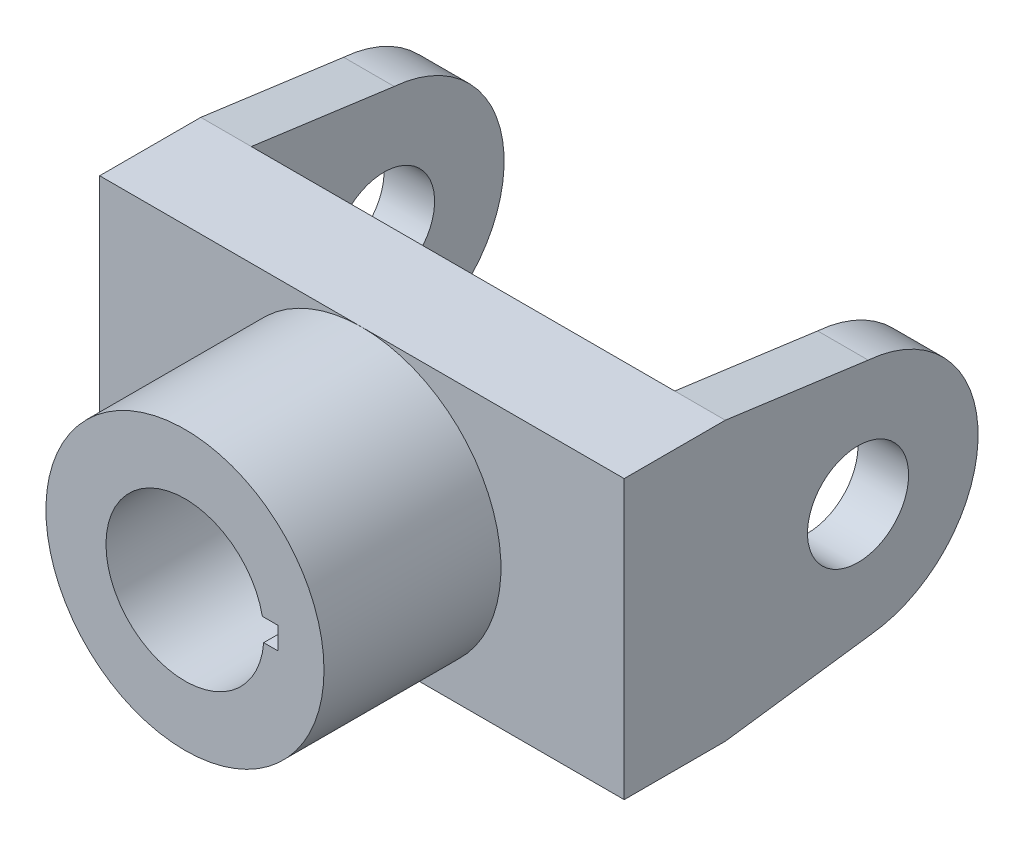
SolidWorks part; units mm, degrees
material "Plain Carbon Steel"
ref_plane "Front Plane" through (0, 0, 0) normal (0, 0, 1) x (1, 0, 0)
ref_plane "Top Plane" through (0, 0, 0) normal (0, 1, 0) x (1, 0, 0)
ref_plane "Right Plane" through (0, 0, 0) normal (1, 0, 0) x (0, 0, -1)
sketch "Base Plate Sketch" plane through (0, 0, 0) normal (0, 0, 1) x (1, 0, 0)
  line L0 (0, 0) -> (83, 0)
  line L1 (83, 0) -> (83, 88)
  line L2 (83, 88) -> (-83, 88)
  line L3 (-83, 88) -> (-83, 0)
  line L4 (-83, 0) -> (0, 0)
  point P6 (-83, 44)
  dimension "D1" = 166
  dimension "D2" = 83
  dimension "D3" = 44
extrude "Base Plate" add sketch "Base Plate Sketch" against normal blind 32
sketch "Fork Arm Sketch" plane through (83, 0, 0) normal (1, 0, 0) x (0, 0, -1)
  line L0 (32, 88) -> (77.2214, 81.8632)
  line L1 (32, 0) -> (77.8924, 6.1999)
  line L2 (32, 0) -> (32, 88)
  arc A0 (77.8924, 6.1999) -> (77.2214, 81.8632) centre (74, 44) ccw
  dimension "D1" = 76
  dimension "D2" = 74
  dimension "D3" = 44
  dimension "D4" = 45.2214
  dimension "D5" = 45.8924
extrude "Fork Arm" add sketch "Fork Arm Sketch" against normal blind 16
mirror "Fork Arm Mirror" about plane through (0, 0, 0) normal (1, 0, 0) of "Fork Arm"
sketch "Hub Sketch" plane through (0, 0, 0) normal (0, 0, 1) x (1, 0, 0)
  circle A0 centre (0, 44) radius 44
  dimension "D1" = 88
  dimension "D2" = 44
extrude "Hub Ø88" add sketch "Hub Sketch" along normal blind 56
sketch "Keyed Bore Sketch" plane through (0, 0, 56) normal (0, 0, 1) x (1, 0, 0)
  line L1 (24.4949, 49) -> (29.4949, 49)
  line L2 (29.4949, 49) -> (29.4949, 42)
  line L3 (29.4949, 42) -> (24.9199, 42)
  arc A0 (24.4949, 49) -> (24.9199, 42) centre (0, 44) ccw
  dimension "D1" = 50
  dimension "D2" = 7
  dimension "D3" = 5
  dimension "D4" = 42
extrude "Keyed Bore Ø50" cut sketch "Keyed Bore Sketch" against normal blind 56
sketch "Pin Hole Sketch" plane through (83, 0, 0) normal (1, 0, 0) x (0, 0, -1)
  circle A0 centre (74, 44) radius 16
  dimension "D1" = 32
extrude "Pin Holes Ø32" cut sketch "Pin Hole Sketch" against normal blind 255
